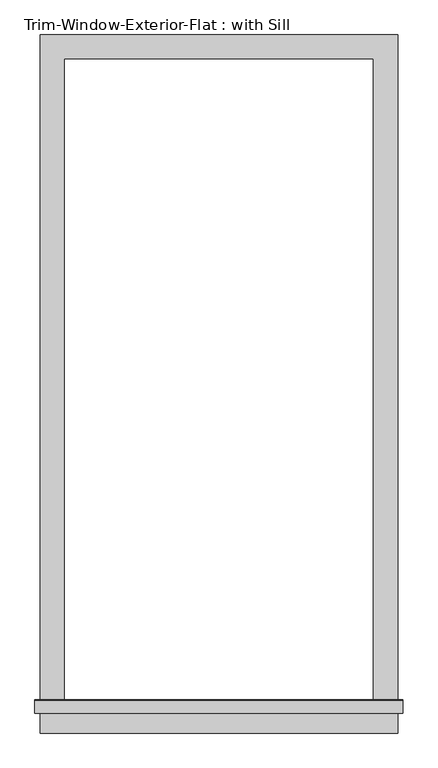
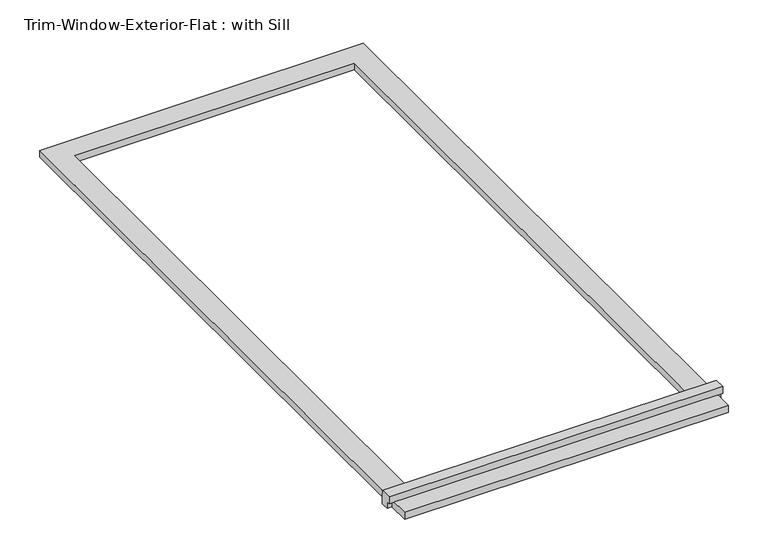
"""IFC4 building model written with IfcOpenShell, lengths in millimetres: proxy geometry, Trim-Window-Exterior-Flat : with Sill."""

from ifc_helpers import new_model, si_unit, frame, origin, origin_with_axes, place, context, project, spatial, polyline, outline, extrude, source, transform, mapped, element, save


def trim_window_exterior_flat_with_sill_683e4a0f(model_context):
    return source(origin(), model_context, "Body", "SweptSolid", [
        extrude(outline(polyline([(425.45, -1546.1823709), (425.45, -1603.3323709), (-425.45, -1603.3323709), (-425.45, -1546.1823709), (425.45, -1546.1823709)])), origin_with_axes(), (0.0, 0.0, 1.0), 19.05),
        extrude(outline(polyline([(-1555.75, 38.1), (-1526.4580645, 38.1), (-1524.0, 19.05), (-1524.0, 0.0), (-1546.1823709, 0.0), (-1546.1823709, 19.05), (-1555.75, 19.05), (-1555.75, 38.1)])), frame((-438.15, 0.0, 0.0), z_axis=(1.0, 0.0, 0.0), x_axis=(0.0, 1.0, 0.0)), (0.0, 0.0, 1.0), 876.3),
        extrude(outline(polyline([(-425.45, 57.15), (425.45, 57.15), (425.45, -1524.0), (368.3, -1524.0), (368.3, 0.0), (-368.3, 0.0), (-368.3, -1524.0), (-425.45, -1524.0), (-425.45, 57.15)])), origin_with_axes(), (0.0, 0.0, 1.0), 19.05),
    ])


if __name__ == "__main__":
    model = new_model("IFC4")
    model_context = context("Model", 3, world=origin())
    ifc_project = project(units=[si_unit("LENGTHUNIT", "METRE", prefix="MILLI")], contexts=[model_context])
    site = spatial("IfcSite", under=ifc_project)
    building = spatial("IfcBuilding", under=site)
    placement = place(None, origin())
    trim_window_exterior_flat_with_sill_shape = trim_window_exterior_flat_with_sill_683e4a0f(model_context)
    element("IfcBuildingElementProxy", 1, Name="Trim-Window-Exterior-Flat : with Sill", ObjectType="Trim-Window-Exterior-Flat : with Sill", at=placement, inside=building, context=model_context, shape_type="MappedRepresentation", body=[
        mapped(trim_window_exterior_flat_with_sill_shape, transform((0.0, 0.0, 0.0), x_axis=(1.0, 0.0, 0.0), y_axis=(0.0, 1.0, 0.0), z_axis=(0.0, 0.0, 1.0))),
    ])
    save(model, "model.ifc")

# Revit data of these elements
# Type "Trim-Window-Exterior-Flat : with Sill"
#   Trim Width = 0' - 2 1/4"
#   Trim Thickness_Picture Frame = 0' - 1 1/4"
#   Trim Thickness_with Sill = 0' - 0 3/4"
#   Sill Thickness = 0' - 1 1/4"
#   Opening Width [instance default] = 2' - 0"
#   Opening Height [instance default] = 3' - 0"
#   Default Elevation = 4' - 0"
#   Sill = yes
#   Picture Frame = no
#   Trim Material [instance default] = none
# Element 1 (IfcBuildingElementProxy, "Trim-Window-Exterior-Flat : with Sill")
#   Opening Width = 2' - 5"
#   Opening Height = 5' - 0"
#   Trim Material = Clad - White
#   Materials on its faces: "Clad - White"
# Materials
#   "Clad - White": class "Wood", colour RGB 242 242 238, transparency 0, Cost = 0
